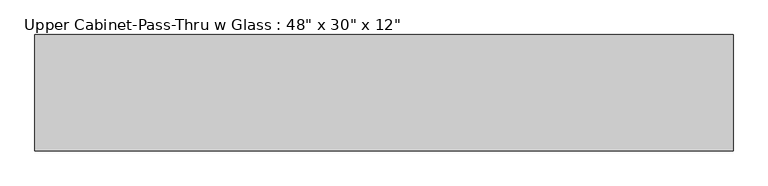
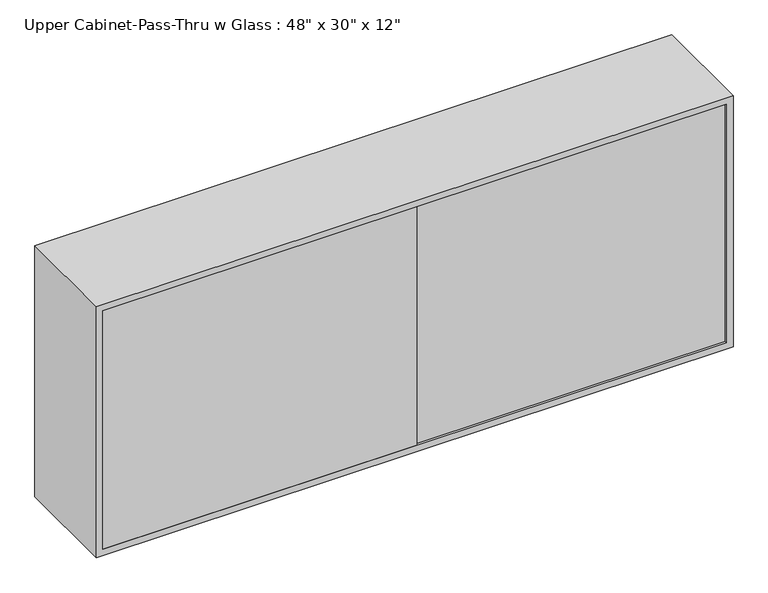
"""IFC4 building model written with IfcOpenShell, lengths in millimetres: furniture geometry."""

from ifc_helpers import new_model, si_unit, frame, origin, place, context, project, spatial, polyline, outline, extrude, source, transform, mapped, element, save


def furniture_1cc80a06(model_context):
    return source(origin(), model_context, "Body", "SweptSolid", [
        extrude(outline(polyline([(1371.6, 933.1377049), (2133.6, 933.1377049), (2133.6, -895.6622951), (1371.6, -895.6622951), (1371.6, 933.1377049)]), holes=[polyline([(1390.65, 914.0877049), (1390.65, -876.6122951), (2114.55, -876.6122951), (2114.55, 914.0877049), (1390.65, 914.0877049)])]), frame((0.0, -304.8, 0.0), z_axis=(0.0, 1.0, 0.0), x_axis=(0.0, 0.0, 1.0)), (0.0, 0.0, 1.0), 304.8),
        extrude(outline(polyline([(25.0877049, -304.8), (-876.6122951, -304.8), (-876.6122951, -298.45), (25.0877049, -298.45), (25.0877049, -304.8)])), frame((0.0, 0.0, 1390.65), z_axis=(0.0, 0.0, 1.0), x_axis=(1.0, 0.0, 0.0)), (0.0, 0.0, 1.0), 723.9),
        extrude(outline(polyline([(914.0877049, -6.35), (12.3877049, -6.35), (12.3877049, 0.0), (914.0877049, 0.0), (914.0877049, -6.35)])), frame((0.0, 0.0, 1390.65), z_axis=(0.0, 0.0, 1.0), x_axis=(1.0, 0.0, 0.0)), (0.0, 0.0, 1.0), 723.9),
        extrude(outline(polyline([(914.0877049, -298.45), (12.3877049, -298.45), (12.3877049, -292.1), (914.0877049, -292.1), (914.0877049, -298.45)])), frame((0.0, 0.0, 1390.65), z_axis=(0.0, 0.0, 1.0), x_axis=(1.0, 0.0, 0.0)), (0.0, 0.0, 1.0), 723.9),
        extrude(outline(polyline([(25.0877049, -12.7), (-876.6122951, -12.7), (-876.6122951, -6.35), (25.0877049, -6.35), (25.0877049, -12.7)])), frame((0.0, 0.0, 1390.65), z_axis=(0.0, 0.0, 1.0), x_axis=(1.0, 0.0, 0.0)), (0.0, 0.0, 1.0), 723.9),
        extrude(outline(polyline([(914.0877049, -285.75), (-876.6122951, -285.75), (-876.6122951, -19.05), (914.0877049, -19.05), (914.0877049, -285.75)])), frame((0.0, 0.0, 1873.25), z_axis=(0.0, 0.0, 1.0), x_axis=(1.0, 0.0, 0.0)), (0.0, 0.0, 1.0), 12.7),
        extrude(outline(polyline([(914.0877049, -285.75), (-876.6122951, -285.75), (-876.6122951, -19.05), (914.0877049, -19.05), (914.0877049, -285.75)])), frame((0.0, 0.0, 1619.25), z_axis=(0.0, 0.0, 1.0), x_axis=(1.0, 0.0, 0.0)), (0.0, 0.0, 1.0), 12.7),
    ])


if __name__ == "__main__":
    model = new_model("IFC4")
    model_context = context("Model", 3, world=origin())
    ifc_project = project(units=[si_unit("LENGTHUNIT", "METRE", prefix="MILLI")], contexts=[model_context])
    site = spatial("IfcSite", under=ifc_project)
    building = spatial("IfcBuilding", under=site)
    placement = place(None, origin())
    furniture_shape = furniture_1cc80a06(model_context)
    element("IfcFurniture", 1, ObjectType="Upper Cabinet-Pass-Thru w Glass : 48\" x 30\" x 12\"", at=placement, inside=building, context=model_context, shape_type="MappedRepresentation", body=[
        mapped(furniture_shape, transform((0.0, 0.0, 0.0), x_axis=(1.0, 0.0, 0.0), y_axis=(0.0, 1.0, 0.0), z_axis=(0.0, 0.0, 1.0))),
    ])
    save(model, "model.ifc")

# Revit data of these elements
# Type "Upper Cabinet-Pass-Thru w Glass : 48\" x 30\" x 12\""
#   Depth = 1' - 0"
#   Height = 2' - 6"
#   Top Of Cabinet = 7' - 0"
#   Width = 6' - 0"
#   Default Elevation = 0
# Element 1 (IfcFurniture, "Upper Cabinet-Pass-Thru w Glass : 48\" x 30\" x 12\"")
#   Materials on its faces: "Glass", "Cabinet"
# Materials
#   "Glass": class "Glass", colour RGB 0 128 192, transparency 0.75, Description = "Soda Lime Glass", Cost = 0
#   "Cabinet": colour RGB 204 122 2, transparency 0
